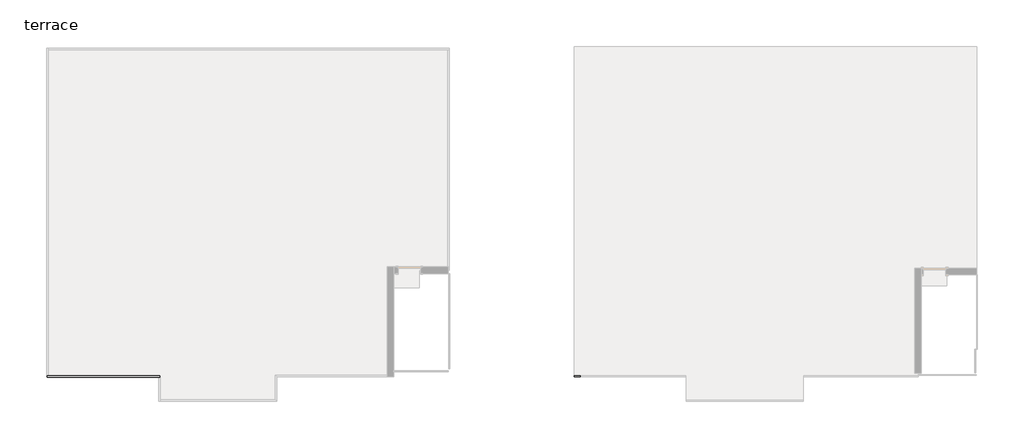
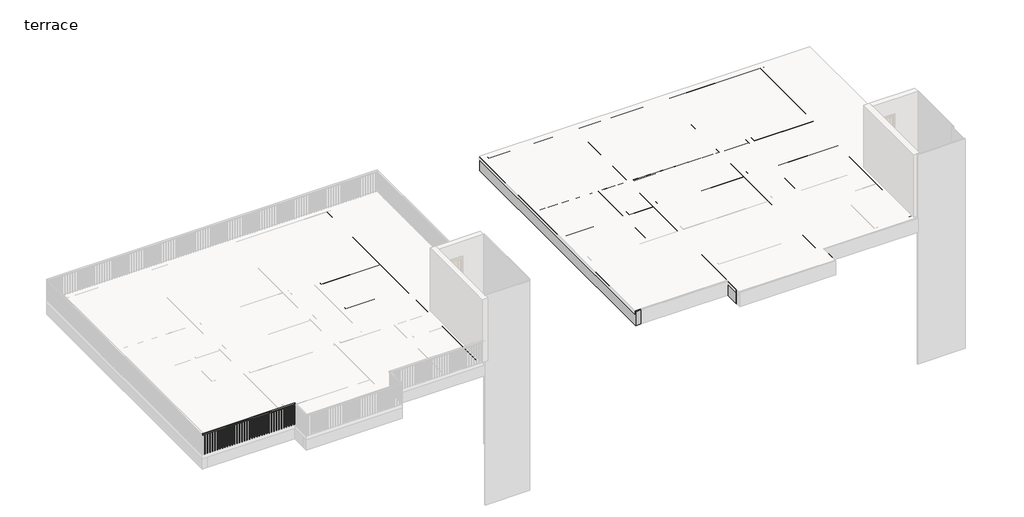
# One storey, part 2 of 6: 17 beams, 1 railing.
"""IFC4 building model written with IfcOpenShell, lengths in millimetres."""

from ifc_helpers import new_model, si_unit, frame, origin, place, context, project, spatial, polyline, outline, extrude, faceted_brep, element, save

model = new_model("IFC4")

# Units and contexts
model_context = context("Model", 3, world=origin())
ifc_project = project(units=[si_unit("LENGTHUNIT", "METRE", prefix="MILLI")], contexts=[model_context])

# Site, building, storey
site = spatial("IfcSite", under=ifc_project)
building = spatial("IfcBuilding", under=site)
storey = spatial("IfcBuildingStorey", under=building, Name="terrace", Elevation=7010.4)

# Beams
placement = place(None, origin())
element("IfcBeam", 1, ObjectType="Concrete-Rectangular Beam", at=placement, inside=storey, context=model_context, shape_type="Brep", body=[
    faceted_brep([(-4641.9993763, 6291.2935985, 7010.4), (-4870.5993763, 6291.2935985, 7010.4), (-4870.5993763, 2709.8935985, 7010.4), (-4870.5993763, 2481.2935985, 7010.4), (-4870.5993763, 957.2935985, 7010.4), (-4870.5993763, 728.6935985, 7010.4), (-4870.5993763, -795.3064015, 7010.4), (-4870.5993763, -1023.9064015, 7010.4), (-4870.5993763, -1785.9064015, 7010.4), (-4870.5993763, -2014.5064015, 7010.4), (-4870.5993763, -4376.7064015, 7010.4), (-4641.9993763, -4376.7064015, 7010.4), (-4870.5993763, 6291.2935985, 6400.8), (-4870.5993763, 2709.8935985, 6400.8), (-4870.5993763, 2481.2935985, 6400.8), (-4870.5993763, 957.2935985, 6400.8), (-4870.5993763, 728.6935985, 6400.8), (-4870.5993763, -795.3064015, 6400.8), (-4870.5993763, -1023.9064015, 6400.8), (-4870.5993763, -1785.9064015, 6400.8), (-4870.5993763, -2014.5064015, 6400.8), (-4870.5993763, -4376.7064015, 6400.8), (-4641.9993763, 6291.2935985, 6400.8), (-4641.9993763, -4376.7064015, 6400.8)], [[[0, 1, 2, 3, 4, 5, 6, 7, 8, 9, 10, 11]], [[1, 12, 13, 14, 15, 16, 17, 18, 19, 20, 21, 10, 9, 8, 7, 6, 5, 4, 3, 2]], [[12, 22, 23, 21, 20, 19, 18, 17, 16, 15, 14, 13]], [[22, 0, 11, 23]], [[1, 0, 22, 12]], [[11, 10, 21, 23]]]),
])
element("IfcBeam", 2, ObjectType="Concrete-Rectangular Beam", at=placement, inside=storey, context=model_context, shape_type="SweptSolid", body=[
    extrude(outline(polyline([(-7308.9993763, 2481.2935985), (-7308.9993763, 2709.8935985), (-4870.5993763, 2709.8935985), (-4870.5993763, 2481.2935985), (-7308.9993763, 2481.2935985)])), frame((0.0, 0.0, 6400.8), z_axis=(0.0, 0.0, 1.0), x_axis=(1.0, 0.0, 0.0)), (0.0, 0.0, 1.0), 609.6),
])
element("IfcBeam", 3, ObjectType="Concrete-Rectangular Beam", at=placement, inside=storey, context=model_context, shape_type="SweptSolid", body=[
    extrude(outline(polyline([(-4870.5993763, 957.2935985), (-4870.5993763, 728.6935985), (-7308.9993763, 728.6935985), (-7308.9993763, 957.2935985), (-4870.5993763, 957.2935985)])), frame((0.0, 0.0, 6400.8), z_axis=(0.0, 0.0, 1.0), x_axis=(1.0, 0.0, 0.0)), (0.0, 0.0, 1.0), 609.6),
])
element("IfcBeam", 4, ObjectType="Concrete-Rectangular Beam", at=placement, inside=storey, context=model_context, shape_type="Brep", body=[
    faceted_brep([(1802.5761273, 6519.8935985, 7010.4), (1573.9761273, 6519.8935985, 7010.4), (1573.9761273, -4605.3064015, 7010.4), (1802.5761273, -4605.3064015, 7010.4), (1802.5761273, -4376.7064015, 7010.4), (1802.5761273, -1023.9064015, 7010.4), (1802.5761273, -795.3064015, 7010.4), (1802.5761273, 728.6935985, 7010.4), (1802.5761273, 957.2935985, 7010.4), (1802.5761273, 2592.6672243, 7010.4), (1802.5761273, 2821.286075, 7010.4), (1802.5761273, 6291.2935985, 7010.4), (1573.9761273, 6519.8935985, 6400.8), (1573.9761273, -4605.3064015, 6400.8), (1802.5761273, 6519.8935985, 6400.8), (1802.5761273, 6291.2935985, 6400.8), (1802.5761273, 2821.286075, 6400.8), (1802.5761273, 2592.6672243, 6400.8), (1802.5761273, 957.2935985, 6400.8), (1802.5761273, 728.6935985, 6400.8), (1802.5761273, -795.3064015, 6400.8), (1802.5761273, -1023.9064015, 6400.8), (1802.5761273, -4376.7064015, 6400.8), (1802.5761273, -4605.3064015, 6400.8)], [[[0, 1, 2, 3, 4, 5, 6, 7, 8, 9, 10, 11]], [[1, 12, 13, 2]], [[12, 14, 15, 16, 17, 18, 19, 20, 21, 22, 23, 13]], [[14, 0, 11, 10, 9, 8, 7, 6, 5, 4, 3, 23, 22, 21, 20, 19, 18, 17, 16, 15]], [[1, 0, 14, 12]], [[3, 2, 13, 23]]]),
])
element("IfcBeam", 5, ObjectType="Concrete-Rectangular Beam", at=placement, inside=storey, context=model_context, shape_type="Brep", body=[
    faceted_brep([(13232.5761273, 6291.2935985, 7010.4), (13232.5761273, 6519.8935985, 7010.4), (1802.5761273, 6519.8935985, 7010.4), (1802.5761273, 6291.2935985, 7010.4), (5383.9761273, 6291.2935985, 7010.4), (5612.5761273, 6291.2935985, 7010.4), (9117.7761273, 6291.2935985, 7010.4), (9346.3761273, 6291.2935985, 7010.4), (13003.9761273, 6291.2935985, 7010.4), (13232.5761273, 6291.2935985, 6400.8), (1802.5761273, 6291.2935985, 6400.8), (5383.9761273, 6291.2935985, 6400.8), (5612.5761273, 6291.2935985, 6400.8), (9117.7761273, 6291.2935985, 6400.8), (9346.3761273, 6291.2935985, 6400.8), (13003.9761273, 6291.2935985, 6400.8), (13232.5761273, 6519.8935985, 6400.8), (1802.5761273, 6519.8935985, 6400.8)], [[[0, 1, 2, 3, 4, 5, 6, 7, 8]], [[9, 0, 8, 7, 6, 5, 4, 3, 10, 11, 12, 13, 14, 15]], [[16, 9, 15, 14, 13, 12, 11, 10, 17]], [[1, 16, 17, 2]], [[3, 2, 17, 10]], [[1, 0, 9, 16]]]),
])
element("IfcBeam", 6, ObjectType="Concrete-Rectangular Beam", at=placement, inside=storey, context=model_context, shape_type="Brep", body=[
    faceted_brep([(5612.5761273, 6291.2935985, 7010.4), (5383.9761273, 6291.2935985, 7010.4), (5383.9761273, 2775.2918938, 7010.4), (5383.9761273, 2546.6730431, 7010.4), (5383.9761273, 957.2935985, 7010.4), (5383.9761273, 728.6935985, 7010.4), (5383.9761273, -795.3064015, 7010.4), (5383.9761273, -1023.9064015, 7010.4), (5383.9761273, -4376.7064015, 7010.4), (5383.9761273, -4605.3064015, 7010.4), (5383.9761273, -5214.9064015, 7010.4), (5612.5761273, -5214.9064015, 7010.4), (5612.5761273, -3538.5064015, 7010.4), (5612.5761273, -3309.9064015, 7010.4), (5612.5761273, -1023.9064015, 7010.4), (5612.5761273, -795.3064015, 7010.4), (5612.5761273, 728.6935985, 7010.4), (5612.5761273, 957.2935985, 7010.4), (5612.5761273, 2481.2935985, 7010.4), (5612.5761273, 2543.7372443, 7010.4), (5612.5761273, 2709.8935985, 7010.4), (5612.5761273, 2772.356095, 7010.4), (5383.9761273, 6291.2935985, 6400.8), (5383.9761273, 2775.2918938, 6400.8), (5383.9761273, 2546.6730431, 6400.8), (5383.9761273, 957.2935985, 6400.8), (5383.9761273, 728.6935985, 6400.8), (5383.9761273, -795.3064015, 6400.8), (5383.9761273, -1023.9064015, 6400.8), (5383.9761273, -4376.7064015, 6400.8), (5383.9761273, -4605.3064015, 6400.8), (5383.9761273, -5214.9064015, 6400.8), (5612.5761273, 6291.2935985, 6400.8), (5612.5761273, 2772.356095, 6400.8), (5612.5761273, 2709.8935985, 6400.8), (5612.5761273, 2543.7372443, 6400.8), (5612.5761273, 2481.2935985, 6400.8), (5612.5761273, 957.2935985, 6400.8), (5612.5761273, 728.6935985, 6400.8), (5612.5761273, -795.3064015, 6400.8), (5612.5761273, -1023.9064015, 6400.8), (5612.5761273, -3309.9064015, 6400.8), (5612.5761273, -3538.5064015, 6400.8), (5612.5761273, -5214.9064015, 6400.8)], [[[0, 1, 2, 3, 4, 5, 6, 7, 8, 9, 10, 11, 12, 13, 14, 15, 16, 17, 18, 19, 20, 21]], [[1, 22, 23, 24, 25, 26, 27, 28, 29, 30, 31, 10, 9, 8, 7, 6, 5, 4, 3, 2]], [[22, 32, 33, 34, 35, 36, 37, 38, 39, 40, 41, 42, 43, 31, 30, 29, 28, 27, 26, 25, 24, 23]], [[32, 0, 21, 20, 19, 18, 17, 16, 15, 14, 13, 12, 11, 43, 42, 41, 40, 39, 38, 37, 36, 35, 34, 33]], [[1, 0, 32, 22]], [[11, 10, 31, 43]]]),
])
element("IfcBeam", 7, ObjectType="Concrete-Rectangular Beam", at=placement, inside=storey, context=model_context, shape_type="Brep", body=[
    faceted_brep([(9117.7761273, -5214.9064015, 7010.4), (9346.3761273, -5214.9064015, 7010.4), (9346.3761273, -4605.3064015, 7010.4), (9346.3761273, -4376.7064015, 7010.4), (9346.3761273, -1023.9064015, 7010.4), (9346.3761273, -795.3064015, 7010.4), (9346.3761273, 728.6935985, 7010.4), (9346.3761273, 957.2935985, 7010.4), (9346.3761273, 2481.2935985, 7010.4), (9346.3761273, 2495.7858639, 7010.4), (9346.3761273, 2709.8935985, 7010.4), (9346.3761273, 2724.4047146, 7010.4), (9346.3761273, 6291.2935985, 7010.4), (9117.7761273, 6291.2935985, 7010.4), (9117.7761273, 2727.3405134, 7010.4), (9117.7761273, 2709.8935985, 7010.4), (9117.7761273, 2498.7216627, 7010.4), (9117.7761273, 2481.2935985, 7010.4), (9117.7761273, 957.2935985, 7010.4), (9117.7761273, 728.6935985, 7010.4), (9117.7761273, -795.3064015, 7010.4), (9117.7761273, -1023.9064015, 7010.4), (9117.7761273, -3309.9064015, 7010.4), (9117.7761273, -3538.5064015, 7010.4), (9346.3761273, -5214.9064015, 6400.8), (9346.3761273, -4605.3064015, 6400.8), (9346.3761273, -4376.7064015, 6400.8), (9346.3761273, -1023.9064015, 6400.8), (9346.3761273, -795.3064015, 6400.8), (9346.3761273, 728.6935985, 6400.8), (9346.3761273, 957.2935985, 6400.8), (9346.3761273, 2481.2935985, 6400.8), (9346.3761273, 2495.7858639, 6400.8), (9346.3761273, 2709.8935985, 6400.8), (9346.3761273, 2724.4047146, 6400.8), (9346.3761273, 6291.2935985, 6400.8), (9117.7761273, -5214.9064015, 6400.8), (9117.7761273, -3538.5064015, 6400.8), (9117.7761273, -3309.9064015, 6400.8), (9117.7761273, -1023.9064015, 6400.8), (9117.7761273, -795.3064015, 6400.8), (9117.7761273, 728.6935985, 6400.8), (9117.7761273, 957.2935985, 6400.8), (9117.7761273, 2481.2935985, 6400.8), (9117.7761273, 2498.7216627, 6400.8), (9117.7761273, 2709.8935985, 6400.8), (9117.7761273, 2727.3405134, 6400.8), (9117.7761273, 6291.2935985, 6400.8)], [[[0, 1, 2, 3, 4, 5, 6, 7, 8, 9, 10, 11, 12, 13, 14, 15, 16, 17, 18, 19, 20, 21, 22, 23]], [[1, 24, 25, 26, 27, 28, 29, 30, 31, 32, 33, 34, 35, 12, 11, 10, 9, 8, 7, 6, 5, 4, 3, 2]], [[24, 36, 37, 38, 39, 40, 41, 42, 43, 44, 45, 46, 47, 35, 34, 33, 32, 31, 30, 29, 28, 27, 26, 25]], [[36, 0, 23, 22, 21, 20, 19, 18, 17, 16, 15, 14, 13, 47, 46, 45, 44, 43, 42, 41, 40, 39, 38, 37]], [[1, 0, 36, 24]], [[13, 12, 35, 47]]]),
])
element("IfcBeam", 8, ObjectType="Concrete-Rectangular Beam", at=placement, inside=storey, context=model_context, shape_type="Brep", body=[
    faceted_brep([(13232.5761273, 6291.2935985, 7010.4), (13003.9761273, 6291.2935985, 7010.4), (13003.9761273, 2709.8935985, 7010.4), (13003.9761273, 2481.2935985, 7010.4), (13003.9761273, 957.2935985, 7010.4), (13003.9761273, 728.6935985, 7010.4), (13003.9761273, -795.3064015, 7010.4), (13003.9761273, -1023.9064015, 7010.4), (13003.9761273, -1785.9064015, 7010.4), (13003.9761273, -2014.5064015, 7010.4), (13003.9761273, -4376.7064015, 7010.4), (13232.5761273, -4376.7064015, 7010.4), (13003.9761273, 6291.2935985, 6400.8), (13003.9761273, 2709.8935985, 6400.8), (13003.9761273, 2481.2935985, 6400.8), (13003.9761273, 957.2935985, 6400.8), (13003.9761273, 728.6935985, 6400.8), (13003.9761273, -795.3064015, 6400.8), (13003.9761273, -1023.9064015, 6400.8), (13003.9761273, -1785.9064015, 6400.8), (13003.9761273, -2014.5064015, 6400.8), (13003.9761273, -4376.7064015, 6400.8), (13232.5761273, 6291.2935985, 6400.8), (13232.5761273, -4376.7064015, 6400.8)], [[[0, 1, 2, 3, 4, 5, 6, 7, 8, 9, 10, 11]], [[1, 12, 13, 14, 15, 16, 17, 18, 19, 20, 21, 10, 9, 8, 7, 6, 5, 4, 3, 2]], [[12, 22, 23, 21, 20, 19, 18, 17, 16, 15, 14, 13]], [[22, 0, 11, 23]], [[1, 0, 22, 12]], [[11, 10, 21, 23]]]),
])
element("IfcBeam", 9, ObjectType="Concrete-Rectangular Beam", at=placement, inside=storey, context=model_context, shape_type="Brep", body=[
    faceted_brep([(10565.5761273, 2709.8935985, 7010.4), (10476.304088, 2709.8935985, 7010.4), (10336.9761273, 2709.8935985, 7010.4), (10336.9761273, 2483.0640691, 7010.4), (10336.9761273, 2481.2935985, 7010.4), (10336.9761273, 957.2935985, 7010.4), (10336.9761273, 728.6935985, 7010.4), (10336.9761273, -795.3064015, 7010.4), (10565.5761273, -795.3064015, 7010.4), (10565.5761273, 728.6935985, 7010.4), (10565.5761273, 957.2935985, 7010.4), (10565.5761273, 2481.2935985, 7010.4), (10565.5761273, 2709.8935985, 6400.8), (10565.5761273, -795.3064015, 6400.8), (10565.5761273, 728.6935985, 6400.8), (10565.5761273, 957.2935985, 6400.8), (10565.5761273, 2481.2935985, 6400.8), (10336.9761273, 2709.8935985, 6400.8), (10476.304088, 2709.8935985, 6400.8), (10336.9761273, -795.3064015, 6400.8), (10336.9761273, 728.6935985, 6400.8), (10336.9761273, 957.2935985, 6400.8), (10336.9761273, 2481.2935985, 6400.8), (10336.9761273, 2483.0640691, 6400.8)], [[[0, 1, 2, 3, 4, 5, 6, 7, 8, 9, 10, 11]], [[12, 0, 11, 10, 9, 8, 13, 14, 15, 16]], [[17, 18, 12, 16, 15, 14, 13, 19, 20, 21, 22, 23]], [[2, 17, 23, 22, 21, 20, 19, 7, 6, 5, 4, 3]], [[8, 7, 19, 13]], [[2, 1, 0, 12, 18, 17]]]),
])
element("IfcBeam", 10, ObjectType="Concrete-Rectangular Beam", at=placement, inside=storey, context=model_context, shape_type="SweptSolid", body=[
    extrude(outline(polyline([(10565.5761273, 2481.2935985), (10565.5761273, 2709.8935985), (13003.9761273, 2709.8935985), (13003.9761273, 2481.2935985), (10565.5761273, 2481.2935985)])), frame((0.0, 0.0, 6400.8), z_axis=(0.0, 0.0, 1.0), x_axis=(1.0, 0.0, 0.0)), (0.0, 0.0, 1.0), 609.6),
])
element("IfcBeam", 11, ObjectType="Concrete-Rectangular Beam", at=placement, inside=storey, context=model_context, shape_type="SweptSolid", body=[
    extrude(outline(polyline([(13003.9761273, 957.2935985), (13003.9761273, 728.6935985), (10565.5761273, 728.6935985), (10565.5761273, 957.2935985), (13003.9761273, 957.2935985)])), frame((0.0, 0.0, 6400.8), z_axis=(0.0, 0.0, 1.0), x_axis=(1.0, 0.0, 0.0)), (0.0, 0.0, 1.0), 609.6),
])
element("IfcBeam", 12, ObjectType="Concrete-Rectangular Beam", at=placement, inside=storey, context=model_context, shape_type="SweptSolid", body=[
    extrude(outline(polyline([(5612.5761273, 2481.2935985), (5612.5761273, 2709.8935985), (9117.7761273, 2709.8935985), (9117.7761273, 2481.2935985), (5612.5761273, 2481.2935985)])), frame((0.0, 0.0, 6400.8), z_axis=(0.0, 0.0, 1.0), x_axis=(1.0, 0.0, 0.0)), (0.0, 0.0, 1.0), 609.6),
    extrude(outline(polyline([(10336.9761273, 2709.8935985), (10336.9761273, 2481.2935985), (9346.3761273, 2481.2935985), (9346.3761273, 2709.8935985), (10336.9761273, 2709.8935985)])), frame((0.0, 0.0, 6400.8), z_axis=(0.0, 0.0, 1.0), x_axis=(1.0, 0.0, 0.0)), (0.0, 0.0, 1.0), 609.6),
])
element("IfcBeam", 13, ObjectType="Concrete-Rectangular Beam", at=placement, inside=storey, context=model_context, shape_type="Brep", body=[
    faceted_brep([(4164.7761273, -795.3064015, 7010.4), (4393.3761273, -795.3064015, 7010.4), (4393.3761273, 728.6935985, 7010.4), (4393.3761273, 957.2935985, 7010.4), (4393.3761273, 2559.3948379, 7010.4), (4164.7761273, 2562.3306367, 7010.4), (4164.7761273, 957.2935985, 7010.4), (4164.7761273, 728.6935985, 7010.4), (4164.7761273, -795.3064015, 6400.8), (4164.7761273, 2562.3306367, 6400.8), (4164.7761273, 957.2935985, 6400.8), (4164.7761273, 728.6935985, 6400.8), (4393.3761273, -795.3064015, 6400.8), (4393.3761273, 2559.3948379, 6400.8), (4393.3761273, 957.2935985, 6400.8), (4393.3761273, 728.6935985, 6400.8)], [[[0, 1, 2, 3, 4, 5, 6, 7]], [[8, 0, 7, 6, 5, 9, 10, 11]], [[12, 8, 11, 10, 9, 13, 14, 15]], [[1, 12, 15, 14, 13, 4, 3, 2]], [[1, 0, 8, 12]], [[5, 4, 13, 9]]]),
])
element("IfcBeam", 14, ObjectType="Concrete-Rectangular Beam", at=placement, inside=storey, context=model_context, shape_type="SweptSolid", body=[
    extrude(outline(polyline([(1802.5761273, 728.6935985), (1802.5761273, 957.2935985), (4164.7761273, 957.2935985), (4164.7761273, 728.6935985), (1802.5761273, 728.6935985)])), frame((0.0, 0.0, 6400.8), z_axis=(0.0, 0.0, 1.0), x_axis=(1.0, 0.0, 0.0)), (0.0, 0.0, 1.0), 609.6),
])
element("IfcBeam", 15, ObjectType="Concrete-Rectangular Beam", at=placement, inside=storey, context=model_context, shape_type="SweptSolid", body=[
    extrude(outline(polyline([(5383.9761273, 957.2935985), (5383.9761273, 728.6935985), (4393.3761273, 728.6935985), (4393.3761273, 957.2935985), (5383.9761273, 957.2935985)])), frame((0.0, 0.0, 6400.8), z_axis=(0.0, 0.0, 1.0), x_axis=(1.0, 0.0, 0.0)), (0.0, 0.0, 1.0), 609.6),
])
element("IfcBeam", 16, ObjectType="Concrete-Rectangular Beam", at=placement, inside=storey, context=model_context, shape_type="SweptSolid", body=[
    extrude(outline(polyline([(5612.5761273, 728.6935985), (5612.5761273, 957.2935985), (9117.7761273, 957.2935985), (9117.7761273, 728.6935985), (5612.5761273, 728.6935985)])), frame((0.0, 0.0, 6400.8), z_axis=(0.0, 0.0, 1.0), x_axis=(1.0, 0.0, 0.0)), (0.0, 0.0, 1.0), 609.6),
    extrude(outline(polyline([(10336.9761273, 957.2935985), (10336.9761273, 728.6935985), (9346.3761273, 728.6935985), (9346.3761273, 957.2935985), (10336.9761273, 957.2935985)])), frame((0.0, 0.0, 6400.8), z_axis=(0.0, 0.0, 1.0), x_axis=(1.0, 0.0, 0.0)), (0.0, 0.0, 1.0), 609.6),
])
element("IfcBeam", 17, ObjectType="Concrete-Rectangular Beam", at=placement, inside=storey, context=model_context, shape_type="Brep", body=[
    faceted_brep([(5383.9761273, 2546.6730431, 7010.4), (5383.9761273, 2775.2918938, 7010.4), (1802.5761273, 2821.286075, 7010.4), (1802.5761273, 2592.6672243, 7010.4), (4164.7761273, 2562.3306367, 7010.4), (4393.3761273, 2559.3948379, 7010.4), (5383.9761273, 2775.2918938, 6400.8), (1802.5761273, 2821.286075, 6400.8), (5383.9761273, 2546.6730431, 6400.8), (4393.3761273, 2559.3948379, 6400.8), (4164.7761273, 2562.3306367, 6400.8), (1802.5761273, 2592.6672243, 6400.8)], [[[0, 1, 2, 3, 4, 5]], [[1, 6, 7, 2]], [[6, 8, 9, 10, 11, 7]], [[8, 0, 5, 4, 3, 11, 10, 9]], [[1, 0, 8, 6]], [[3, 2, 7, 11]]]),
    faceted_brep([(10336.9761273, 2709.8935985, 7010.4), (10336.9761273, 2483.0640691, 7010.4), (10336.9761273, 2483.0640691, 6400.8), (10336.9761273, 2709.8935985, 6400.8), (10476.304088, 2709.8935985, 6400.8), (10476.304088, 2709.8935985, 7010.4), (9346.3761273, 2495.7858639, 7010.4), (9346.3761273, 2724.4047146, 7010.4), (9346.3761273, 2724.4047146, 6400.8), (9346.3761273, 2495.7858639, 6400.8)], [[[0, 1, 2, 3]], [[0, 3, 4, 5]], [[6, 7, 8, 9]], [[1, 0, 5, 7, 6]], [[5, 4, 8, 7]], [[3, 2, 9, 8, 4]], [[2, 1, 6, 9]]]),
    faceted_brep([(5612.5761273, 2543.7372443, 7010.4), (5612.5761273, 2772.356095, 7010.4), (5612.5761273, 2772.356095, 6400.8), (5612.5761273, 2543.7372443, 6400.8), (9117.7761273, 2498.7216627, 7010.4), (9117.7761273, 2727.3405134, 7010.4), (9117.7761273, 2727.3405134, 6400.8), (9117.7761273, 2498.7216627, 6400.8)], [[[0, 1, 2, 3]], [[1, 0, 4, 5]], [[2, 1, 5, 6]], [[3, 2, 6, 7]], [[0, 3, 7, 4]], [[5, 4, 7, 6]]]),
])

# Railing
element("IfcRailing", 18, ObjectType="Handrail - Rectangular", at=placement, inside=storey, context=model_context, shape_type="SweptSolid", body=[
    extrude(outline(polyline([(-16281.5493763, -4618.0064015), (-16281.5493763, -4567.2064015), (-12471.5493763, -4567.2064015), (-12471.5493763, -4618.0064015), (-16281.5493763, -4618.0064015)])), frame((0.0, 0.0, 7874.0), z_axis=(0.0, 0.0, 1.0), x_axis=(1.0, 0.0, 0.0)), (0.0, 0.0, 1.0), 50.8),
    extrude(outline(polyline([(-12531.8743763, -4602.1314015), (-12531.8743763, -4583.0814015), (-12512.8243763, -4583.0814015), (-12512.8243763, -4602.1314015), (-12531.8743763, -4602.1314015)])), frame((0.0, 0.0, 7010.4), z_axis=(0.0, 0.0, 1.0), x_axis=(1.0, 0.0, 0.0)), (0.0, 0.0, 1.0), 863.6),
    extrude(outline(polyline([(-12633.4743763, -4602.1314015), (-12633.4743763, -4583.0814015), (-12614.4243763, -4583.0814015), (-12614.4243763, -4602.1314015), (-12633.4743763, -4602.1314015)])), frame((0.0, 0.0, 7010.4), z_axis=(0.0, 0.0, 1.0), x_axis=(1.0, 0.0, 0.0)), (0.0, 0.0, 1.0), 863.6),
    extrude(outline(polyline([(-12735.0743763, -4602.1314015), (-12735.0743763, -4583.0814015), (-12716.0243763, -4583.0814015), (-12716.0243763, -4602.1314015), (-12735.0743763, -4602.1314015)])), frame((0.0, 0.0, 7010.4), z_axis=(0.0, 0.0, 1.0), x_axis=(1.0, 0.0, 0.0)), (0.0, 0.0, 1.0), 863.6),
    extrude(outline(polyline([(-12836.6743763, -4602.1314015), (-12836.6743763, -4583.0814015), (-12817.6243763, -4583.0814015), (-12817.6243763, -4602.1314015), (-12836.6743763, -4602.1314015)])), frame((0.0, 0.0, 7010.4), z_axis=(0.0, 0.0, 1.0), x_axis=(1.0, 0.0, 0.0)), (0.0, 0.0, 1.0), 863.6),
    extrude(outline(polyline([(-12938.2743763, -4602.1314015), (-12938.2743763, -4583.0814015), (-12919.2243763, -4583.0814015), (-12919.2243763, -4602.1314015), (-12938.2743763, -4602.1314015)])), frame((0.0, 0.0, 7010.4), z_axis=(0.0, 0.0, 1.0), x_axis=(1.0, 0.0, 0.0)), (0.0, 0.0, 1.0), 863.6),
    extrude(outline(polyline([(-13039.8743763, -4602.1314015), (-13039.8743763, -4583.0814015), (-13020.8243763, -4583.0814015), (-13020.8243763, -4602.1314015), (-13039.8743763, -4602.1314015)])), frame((0.0, 0.0, 7010.4), z_axis=(0.0, 0.0, 1.0), x_axis=(1.0, 0.0, 0.0)), (0.0, 0.0, 1.0), 863.6),
    extrude(outline(polyline([(-13141.4743763, -4602.1314015), (-13141.4743763, -4583.0814015), (-13122.4243763, -4583.0814015), (-13122.4243763, -4602.1314015), (-13141.4743763, -4602.1314015)])), frame((0.0, 0.0, 7010.4), z_axis=(0.0, 0.0, 1.0), x_axis=(1.0, 0.0, 0.0)), (0.0, 0.0, 1.0), 863.6),
    extrude(outline(polyline([(-13243.0743763, -4602.1314015), (-13243.0743763, -4583.0814015), (-13224.0243763, -4583.0814015), (-13224.0243763, -4602.1314015), (-13243.0743763, -4602.1314015)])), frame((0.0, 0.0, 7010.4), z_axis=(0.0, 0.0, 1.0), x_axis=(1.0, 0.0, 0.0)), (0.0, 0.0, 1.0), 863.6),
    extrude(outline(polyline([(-13344.6743763, -4602.1314015), (-13344.6743763, -4583.0814015), (-13325.6243763, -4583.0814015), (-13325.6243763, -4602.1314015), (-13344.6743763, -4602.1314015)])), frame((0.0, 0.0, 7010.4), z_axis=(0.0, 0.0, 1.0), x_axis=(1.0, 0.0, 0.0)), (0.0, 0.0, 1.0), 863.6),
    extrude(outline(polyline([(-13446.2743763, -4602.1314015), (-13446.2743763, -4583.0814015), (-13427.2243763, -4583.0814015), (-13427.2243763, -4602.1314015), (-13446.2743763, -4602.1314015)])), frame((0.0, 0.0, 7010.4), z_axis=(0.0, 0.0, 1.0), x_axis=(1.0, 0.0, 0.0)), (0.0, 0.0, 1.0), 863.6),
    extrude(outline(polyline([(-13547.8743763, -4602.1314015), (-13547.8743763, -4583.0814015), (-13528.8243763, -4583.0814015), (-13528.8243763, -4602.1314015), (-13547.8743763, -4602.1314015)])), frame((0.0, 0.0, 7010.4), z_axis=(0.0, 0.0, 1.0), x_axis=(1.0, 0.0, 0.0)), (0.0, 0.0, 1.0), 863.6),
    extrude(outline(polyline([(-13649.4743763, -4602.1314015), (-13649.4743763, -4583.0814015), (-13630.4243763, -4583.0814015), (-13630.4243763, -4602.1314015), (-13649.4743763, -4602.1314015)])), frame((0.0, 0.0, 7010.4), z_axis=(0.0, 0.0, 1.0), x_axis=(1.0, 0.0, 0.0)), (0.0, 0.0, 1.0), 863.6),
    extrude(outline(polyline([(-13751.0743763, -4602.1314015), (-13751.0743763, -4583.0814015), (-13732.0243763, -4583.0814015), (-13732.0243763, -4602.1314015), (-13751.0743763, -4602.1314015)])), frame((0.0, 0.0, 7010.4), z_axis=(0.0, 0.0, 1.0), x_axis=(1.0, 0.0, 0.0)), (0.0, 0.0, 1.0), 863.6),
    extrude(outline(polyline([(-13852.6743763, -4602.1314015), (-13852.6743763, -4583.0814015), (-13833.6243763, -4583.0814015), (-13833.6243763, -4602.1314015), (-13852.6743763, -4602.1314015)])), frame((0.0, 0.0, 7010.4), z_axis=(0.0, 0.0, 1.0), x_axis=(1.0, 0.0, 0.0)), (0.0, 0.0, 1.0), 863.6),
    extrude(outline(polyline([(-13954.2743763, -4602.1314015), (-13954.2743763, -4583.0814015), (-13935.2243763, -4583.0814015), (-13935.2243763, -4602.1314015), (-13954.2743763, -4602.1314015)])), frame((0.0, 0.0, 7010.4), z_axis=(0.0, 0.0, 1.0), x_axis=(1.0, 0.0, 0.0)), (0.0, 0.0, 1.0), 863.6),
    extrude(outline(polyline([(-14055.8743763, -4602.1314015), (-14055.8743763, -4583.0814015), (-14036.8243763, -4583.0814015), (-14036.8243763, -4602.1314015), (-14055.8743763, -4602.1314015)])), frame((0.0, 0.0, 7010.4), z_axis=(0.0, 0.0, 1.0), x_axis=(1.0, 0.0, 0.0)), (0.0, 0.0, 1.0), 863.6),
    extrude(outline(polyline([(-14157.4743763, -4602.1314015), (-14157.4743763, -4583.0814015), (-14138.4243763, -4583.0814015), (-14138.4243763, -4602.1314015), (-14157.4743763, -4602.1314015)])), frame((0.0, 0.0, 7010.4), z_axis=(0.0, 0.0, 1.0), x_axis=(1.0, 0.0, 0.0)), (0.0, 0.0, 1.0), 863.6),
    extrude(outline(polyline([(-14259.0743763, -4602.1314015), (-14259.0743763, -4583.0814015), (-14240.0243763, -4583.0814015), (-14240.0243763, -4602.1314015), (-14259.0743763, -4602.1314015)])), frame((0.0, 0.0, 7010.4), z_axis=(0.0, 0.0, 1.0), x_axis=(1.0, 0.0, 0.0)), (0.0, 0.0, 1.0), 863.6),
    extrude(outline(polyline([(-14360.6743763, -4602.1314015), (-14360.6743763, -4583.0814015), (-14341.6243763, -4583.0814015), (-14341.6243763, -4602.1314015), (-14360.6743763, -4602.1314015)])), frame((0.0, 0.0, 7010.4), z_axis=(0.0, 0.0, 1.0), x_axis=(1.0, 0.0, 0.0)), (0.0, 0.0, 1.0), 863.6),
    extrude(outline(polyline([(-14462.2743763, -4602.1314015), (-14462.2743763, -4583.0814015), (-14443.2243763, -4583.0814015), (-14443.2243763, -4602.1314015), (-14462.2743763, -4602.1314015)])), frame((0.0, 0.0, 7010.4), z_axis=(0.0, 0.0, 1.0), x_axis=(1.0, 0.0, 0.0)), (0.0, 0.0, 1.0), 863.6),
    extrude(outline(polyline([(-14563.8743763, -4602.1314015), (-14563.8743763, -4583.0814015), (-14544.8243763, -4583.0814015), (-14544.8243763, -4602.1314015), (-14563.8743763, -4602.1314015)])), frame((0.0, 0.0, 7010.4), z_axis=(0.0, 0.0, 1.0), x_axis=(1.0, 0.0, 0.0)), (0.0, 0.0, 1.0), 863.6),
    extrude(outline(polyline([(-14665.4743763, -4602.1314015), (-14665.4743763, -4583.0814015), (-14646.4243763, -4583.0814015), (-14646.4243763, -4602.1314015), (-14665.4743763, -4602.1314015)])), frame((0.0, 0.0, 7010.4), z_axis=(0.0, 0.0, 1.0), x_axis=(1.0, 0.0, 0.0)), (0.0, 0.0, 1.0), 863.6),
    extrude(outline(polyline([(-14767.0743763, -4602.1314015), (-14767.0743763, -4583.0814015), (-14748.0243763, -4583.0814015), (-14748.0243763, -4602.1314015), (-14767.0743763, -4602.1314015)])), frame((0.0, 0.0, 7010.4), z_axis=(0.0, 0.0, 1.0), x_axis=(1.0, 0.0, 0.0)), (0.0, 0.0, 1.0), 863.6),
    extrude(outline(polyline([(-14868.6743763, -4602.1314015), (-14868.6743763, -4583.0814015), (-14849.6243763, -4583.0814015), (-14849.6243763, -4602.1314015), (-14868.6743763, -4602.1314015)])), frame((0.0, 0.0, 7010.4), z_axis=(0.0, 0.0, 1.0), x_axis=(1.0, 0.0, 0.0)), (0.0, 0.0, 1.0), 863.6),
    extrude(outline(polyline([(-14970.2743763, -4602.1314015), (-14970.2743763, -4583.0814015), (-14951.2243763, -4583.0814015), (-14951.2243763, -4602.1314015), (-14970.2743763, -4602.1314015)])), frame((0.0, 0.0, 7010.4), z_axis=(0.0, 0.0, 1.0), x_axis=(1.0, 0.0, 0.0)), (0.0, 0.0, 1.0), 863.6),
    extrude(outline(polyline([(-15071.8743763, -4602.1314015), (-15071.8743763, -4583.0814015), (-15052.8243763, -4583.0814015), (-15052.8243763, -4602.1314015), (-15071.8743763, -4602.1314015)])), frame((0.0, 0.0, 7010.4), z_axis=(0.0, 0.0, 1.0), x_axis=(1.0, 0.0, 0.0)), (0.0, 0.0, 1.0), 863.6),
    extrude(outline(polyline([(-15173.4743763, -4602.1314015), (-15173.4743763, -4583.0814015), (-15154.4243763, -4583.0814015), (-15154.4243763, -4602.1314015), (-15173.4743763, -4602.1314015)])), frame((0.0, 0.0, 7010.4), z_axis=(0.0, 0.0, 1.0), x_axis=(1.0, 0.0, 0.0)), (0.0, 0.0, 1.0), 863.6),
    extrude(outline(polyline([(-15275.0743763, -4602.1314015), (-15275.0743763, -4583.0814015), (-15256.0243763, -4583.0814015), (-15256.0243763, -4602.1314015), (-15275.0743763, -4602.1314015)])), frame((0.0, 0.0, 7010.4), z_axis=(0.0, 0.0, 1.0), x_axis=(1.0, 0.0, 0.0)), (0.0, 0.0, 1.0), 863.6),
    extrude(outline(polyline([(-15376.6743763, -4602.1314015), (-15376.6743763, -4583.0814015), (-15357.6243763, -4583.0814015), (-15357.6243763, -4602.1314015), (-15376.6743763, -4602.1314015)])), frame((0.0, 0.0, 7010.4), z_axis=(0.0, 0.0, 1.0), x_axis=(1.0, 0.0, 0.0)), (0.0, 0.0, 1.0), 863.6),
    extrude(outline(polyline([(-15478.2743763, -4602.1314015), (-15478.2743763, -4583.0814015), (-15459.2243763, -4583.0814015), (-15459.2243763, -4602.1314015), (-15478.2743763, -4602.1314015)])), frame((0.0, 0.0, 7010.4), z_axis=(0.0, 0.0, 1.0), x_axis=(1.0, 0.0, 0.0)), (0.0, 0.0, 1.0), 863.6),
    extrude(outline(polyline([(-15579.8743763, -4602.1314015), (-15579.8743763, -4583.0814015), (-15560.8243763, -4583.0814015), (-15560.8243763, -4602.1314015), (-15579.8743763, -4602.1314015)])), frame((0.0, 0.0, 7010.4), z_axis=(0.0, 0.0, 1.0), x_axis=(1.0, 0.0, 0.0)), (0.0, 0.0, 1.0), 863.6),
    extrude(outline(polyline([(-15681.4743763, -4602.1314015), (-15681.4743763, -4583.0814015), (-15662.4243763, -4583.0814015), (-15662.4243763, -4602.1314015), (-15681.4743763, -4602.1314015)])), frame((0.0, 0.0, 7010.4), z_axis=(0.0, 0.0, 1.0), x_axis=(1.0, 0.0, 0.0)), (0.0, 0.0, 1.0), 863.6),
    extrude(outline(polyline([(-15783.0743763, -4602.1314015), (-15783.0743763, -4583.0814015), (-15764.0243763, -4583.0814015), (-15764.0243763, -4602.1314015), (-15783.0743763, -4602.1314015)])), frame((0.0, 0.0, 7010.4), z_axis=(0.0, 0.0, 1.0), x_axis=(1.0, 0.0, 0.0)), (0.0, 0.0, 1.0), 863.6),
    extrude(outline(polyline([(-15884.6743763, -4602.1314015), (-15884.6743763, -4583.0814015), (-15865.6243763, -4583.0814015), (-15865.6243763, -4602.1314015), (-15884.6743763, -4602.1314015)])), frame((0.0, 0.0, 7010.4), z_axis=(0.0, 0.0, 1.0), x_axis=(1.0, 0.0, 0.0)), (0.0, 0.0, 1.0), 863.6),
    extrude(outline(polyline([(-15986.2743763, -4602.1314015), (-15986.2743763, -4583.0814015), (-15967.2243763, -4583.0814015), (-15967.2243763, -4602.1314015), (-15986.2743763, -4602.1314015)])), frame((0.0, 0.0, 7010.4), z_axis=(0.0, 0.0, 1.0), x_axis=(1.0, 0.0, 0.0)), (0.0, 0.0, 1.0), 863.6),
    extrude(outline(polyline([(-16087.8743763, -4602.1314015), (-16087.8743763, -4583.0814015), (-16068.8243763, -4583.0814015), (-16068.8243763, -4602.1314015), (-16087.8743763, -4602.1314015)])), frame((0.0, 0.0, 7010.4), z_axis=(0.0, 0.0, 1.0), x_axis=(1.0, 0.0, 0.0)), (0.0, 0.0, 1.0), 863.6),
    extrude(outline(polyline([(-16189.4743763, -4602.1314015), (-16189.4743763, -4583.0814015), (-16170.4243763, -4583.0814015), (-16170.4243763, -4602.1314015), (-16189.4743763, -4602.1314015)])), frame((0.0, 0.0, 7010.4), z_axis=(0.0, 0.0, 1.0), x_axis=(1.0, 0.0, 0.0)), (0.0, 0.0, 1.0), 863.6),
    extrude(outline(polyline([(-12490.5993763, -4602.1314015), (-12490.5993763, -4583.0814015), (-12471.5493763, -4583.0814015), (-12471.5493763, -4602.1314015), (-12490.5993763, -4602.1314015)])), frame((0.0, 0.0, 7010.4), z_axis=(0.0, 0.0, 1.0), x_axis=(1.0, 0.0, 0.0)), (0.0, 0.0, 1.0), 863.6),
    extrude(outline(polyline([(-16281.5493763, -4602.1314015), (-16281.5493763, -4583.0814015), (-16262.4993763, -4583.0814015), (-16262.4993763, -4602.1314015), (-16281.5493763, -4602.1314015)])), frame((0.0, 0.0, 7010.4), z_axis=(0.0, 0.0, 1.0), x_axis=(1.0, 0.0, 0.0)), (0.0, 0.0, 1.0), 863.6),
])

save(model, "model.ifc")

# Revit data of these elements
# Type "Concrete-Rectangular Beam"
#   Assembly Code = "B10"
#   Length [instance default] = 5' - 0"
#   b = 0' - 9"
#   h = 2' - 0"
#   Structural Material [instance default] = Concrete, Cast-in-Place gray
# Type "Handrail - Rectangular"
#   Assembly Code = "C2010400"
#   built-in parameter 1008612 = 0.0416667 (stored number, unit not read)
#   built-in parameter 1008611 = 0.0416667 (stored number, unit not read)
#   built-in parameter 1008609 = 0.333333 (stored number, unit not read)
#   built-in parameter 1008604 = 0.166667 (stored number, unit not read)
#   built-in parameter 1008603 = 0.166667 (stored number, unit not read)
#   Railing Height = 3' - 0"
#   built-in parameter 1008630 = 2
#   built-in parameter 1008610 = 2
#   built-in parameter 1008618 = Baluster - Square : 3/4"
# Elements 1, 2, 3, 4, 5, 6, 7, 8, 9, 10, 11, 12, 13, 14, 15, 16, 17 (IfcBeam, "Concrete-Rectangular Beam")
#   Structural Material = Concrete, Cast-in-Place gray
#   Phase Created = New Construction
#   Materials on its faces: "Concrete, Cast-in-Place gray"
# Element 18 (IfcRailing, "Handrail - Rectangular")
#   Phase Created = New Construction
# Materials
#   "Concrete, Cast-in-Place gray": class "Concrete", colour RGB 192 192 192, transparency 0, Description = "Cast-in-place concrete", Cost = 0
